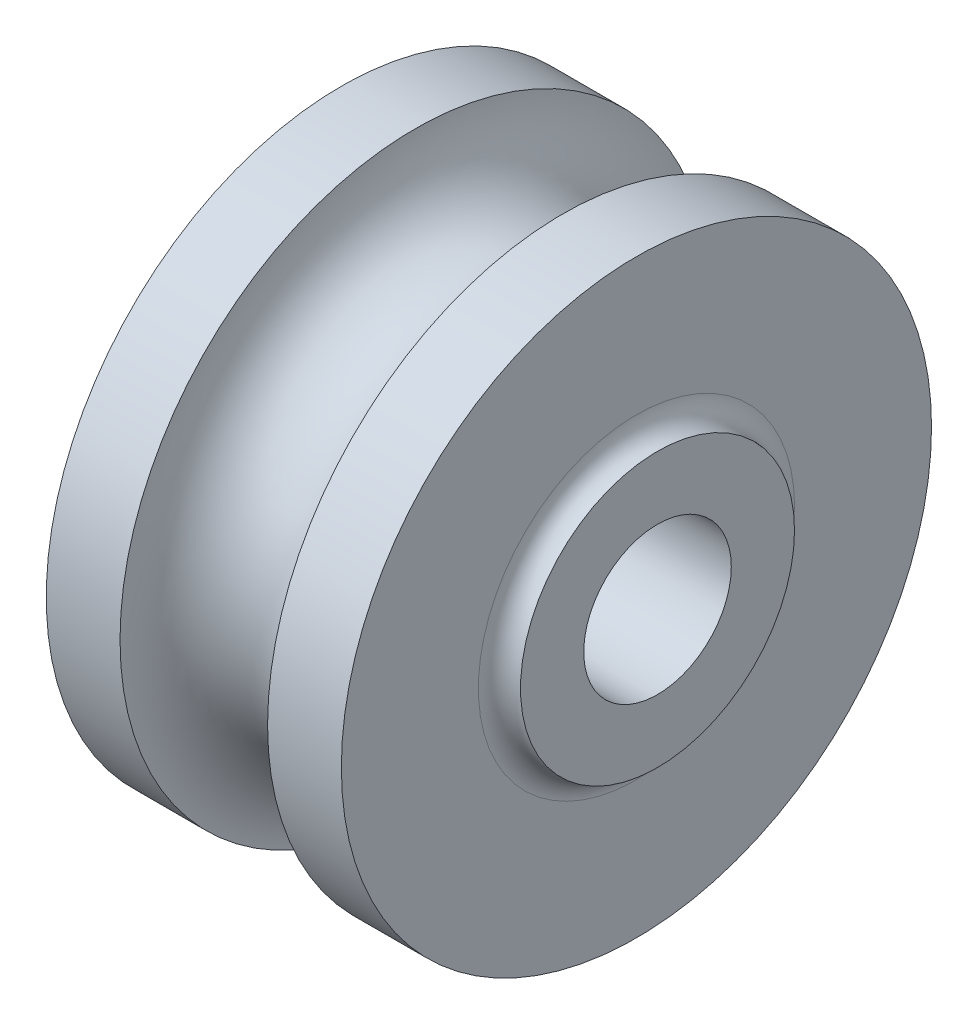
ISO-10303-21;
HEADER;
FILE_DESCRIPTION(('STEP AP214'),'2;1');
FILE_NAME('part.step','',(''),(''),'','','');
FILE_SCHEMA(('AUTOMOTIVE_DESIGN { 1 0 10303 214 1 1 1 1 }'));
ENDSEC;
DATA;
#1=APPLICATION_CONTEXT('core data for automotive mechanical design processes');
#2=APPLICATION_PROTOCOL_DEFINITION('international standard','automotive_design',2000,#1);
#3=PRODUCT_CONTEXT('',#1,'mechanical');
#4=PRODUCT('Part','Part','',(#3));
#5=PRODUCT_RELATED_PRODUCT_CATEGORY('part','',(#4));
#6=PRODUCT_DEFINITION_FORMATION('','',#4);
#7=PRODUCT_DEFINITION_CONTEXT('part definition',#1,'design');
#8=PRODUCT_DEFINITION('design','',#6,#7);
#9=PRODUCT_DEFINITION_SHAPE('','',#8);
#10=(LENGTH_UNIT() NAMED_UNIT(*) SI_UNIT(.MILLI.,.METRE.));
#11=(NAMED_UNIT(*) PLANE_ANGLE_UNIT() SI_UNIT($,.RADIAN.));
#12=(NAMED_UNIT(*) SI_UNIT($,.STERADIAN.) SOLID_ANGLE_UNIT());
#13=UNCERTAINTY_MEASURE_WITH_UNIT(LENGTH_MEASURE(1.E-05),#10,'distance_accuracy_value','');
#14=(GEOMETRIC_REPRESENTATION_CONTEXT(3) GLOBAL_UNCERTAINTY_ASSIGNED_CONTEXT((#13)) GLOBAL_UNIT_ASSIGNED_CONTEXT((#10,
#11,#12)) REPRESENTATION_CONTEXT('',''));
#15=CARTESIAN_POINT('',(0.,0.,0.));
#16=DIRECTION('',(0.,0.,1.));
#17=DIRECTION('',(1.,0.,0.));
#18=AXIS2_PLACEMENT_3D('',#15,#16,#17);
#19=CARTESIAN_POINT('',(14.,0.,0.));
#20=DIRECTION('',(-1.,0.,0.));
#21=DIRECTION('',(0.,0.,1.));
#22=AXIS2_PLACEMENT_3D('',#19,#20,#21);
#23=CYLINDRICAL_SURFACE('',#22,28.);
#24=CARTESIAN_POINT('',(-14.,0.,0.));
#25=DIRECTION('',(1.,0.,0.));
#26=DIRECTION('',(0.,0.,-1.));
#27=AXIS2_PLACEMENT_3D('',#24,#25,#26);
#28=CIRCLE('',#27,28.);
#29=CARTESIAN_POINT('',(-14.,0.,-28.));
#30=VERTEX_POINT('',#29);
#31=EDGE_CURVE('E78',#30,#30,#28,.T.);
#32=ORIENTED_EDGE('',*,*,#31,.T.);
#33=EDGE_LOOP('',(#32));
#34=FACE_BOUND('',#33,.T.);
#35=CARTESIAN_POINT('',(-7.,0.,0.));
#36=DIRECTION('',(1.,0.,0.));
#37=DIRECTION('',(0.,0.,-1.));
#38=AXIS2_PLACEMENT_3D('',#35,#36,#37);
#39=CIRCLE('',#38,28.);
#40=CARTESIAN_POINT('',(-7.,0.,-28.));
#41=VERTEX_POINT('',#40);
#42=EDGE_CURVE('E43',#41,#41,#39,.T.);
#43=ORIENTED_EDGE('',*,*,#42,.F.);
#44=EDGE_LOOP('',(#43));
#45=FACE_BOUND('',#44,.T.);
#46=ADVANCED_FACE('F39',(#34,#45),#23,.T.);
#47=CARTESIAN_POINT('',(14.,0.,0.));
#48=DIRECTION('',(1.,0.,0.));
#49=DIRECTION('',(0.,0.,-1.));
#50=AXIS2_PLACEMENT_3D('',#47,#48,#49);
#51=CIRCLE('',#50,28.);
#52=CARTESIAN_POINT('',(14.,0.,-28.));
#53=VERTEX_POINT('',#52);
#54=EDGE_CURVE('E55',#53,#53,#51,.T.);
#55=ORIENTED_EDGE('',*,*,#54,.F.);
#56=EDGE_LOOP('',(#55));
#57=FACE_BOUND('',#56,.T.);
#58=CARTESIAN_POINT('',(7.,0.,0.));
#59=DIRECTION('',(-1.,0.,0.));
#60=DIRECTION('',(0.,0.,1.));
#61=AXIS2_PLACEMENT_3D('',#58,#59,#60);
#62=CIRCLE('',#61,28.);
#63=CARTESIAN_POINT('',(7.,0.,28.));
#64=VERTEX_POINT('',#63);
#65=EDGE_CURVE('E54',#64,#64,#62,.T.);
#66=ORIENTED_EDGE('',*,*,#65,.F.);
#67=EDGE_LOOP('',(#66));
#68=FACE_BOUND('',#67,.T.);
#69=ADVANCED_FACE('F102',(#57,#68),#23,.T.);
#70=CARTESIAN_POINT('',(14.,0.,0.));
#71=DIRECTION('',(1.,0.,0.));
#72=DIRECTION('',(0.,0.,-1.));
#73=AXIS2_PLACEMENT_3D('',#70,#71,#72);
#74=PLANE('',#73);
#75=CARTESIAN_POINT('',(14.,0.,0.));
#76=DIRECTION('',(1.,0.,0.));
#77=DIRECTION('',(0.,0.,-1.));
#78=AXIS2_PLACEMENT_3D('',#75,#76,#77);
#79=CIRCLE('',#78,15.);
#80=CARTESIAN_POINT('',(14.,0.,-15.));
#81=VERTEX_POINT('',#80);
#82=EDGE_CURVE('E50',#81,#81,#79,.F.);
#83=ORIENTED_EDGE('',*,*,#82,.T.);
#84=EDGE_LOOP('',(#83));
#85=FACE_BOUND('',#84,.T.);
#86=ORIENTED_EDGE('',*,*,#54,.T.);
#87=EDGE_LOOP('',(#86));
#88=FACE_BOUND('',#87,.T.);
#89=ADVANCED_FACE('F109',(#85,#88),#74,.T.);
#90=CARTESIAN_POINT('',(-14.,0.,0.));
#91=DIRECTION('',(1.,0.,0.));
#92=DIRECTION('',(0.,0.,-1.));
#93=AXIS2_PLACEMENT_3D('',#90,#91,#92);
#94=PLANE('',#93);
#95=CARTESIAN_POINT('',(-14.,0.,0.));
#96=DIRECTION('',(1.,0.,0.));
#97=DIRECTION('',(0.,0.,-1.));
#98=AXIS2_PLACEMENT_3D('',#95,#96,#97);
#99=CIRCLE('',#98,15.);
#100=CARTESIAN_POINT('',(-14.,0.,-15.));
#101=VERTEX_POINT('',#100);
#102=EDGE_CURVE('E10',#101,#101,#99,.T.);
#103=ORIENTED_EDGE('',*,*,#102,.T.);
#104=EDGE_LOOP('',(#103));
#105=FACE_BOUND('',#104,.T.);
#106=ORIENTED_EDGE('',*,*,#31,.F.);
#107=EDGE_LOOP('',(#106));
#108=FACE_BOUND('',#107,.T.);
#109=ADVANCED_FACE('F111',(#105,#108),#94,.F.);
#110=CARTESIAN_POINT('',(-16.,0.,0.));
#111=DIRECTION('',(1.,0.,0.));
#112=DIRECTION('',(0.,0.,-1.));
#113=AXIS2_PLACEMENT_3D('',#110,#111,#112);
#114=PLANE('',#113);
#115=CARTESIAN_POINT('',(-16.,0.,0.));
#116=DIRECTION('',(1.,0.,0.));
#117=DIRECTION('',(0.,0.,-1.));
#118=AXIS2_PLACEMENT_3D('',#115,#116,#117);
#119=CIRCLE('',#118,7.);
#120=CARTESIAN_POINT('',(-16.,0.,-7.));
#121=VERTEX_POINT('',#120);
#122=EDGE_CURVE('E58',#121,#121,#119,.T.);
#123=ORIENTED_EDGE('',*,*,#122,.T.);
#124=EDGE_LOOP('',(#123));
#125=FACE_BOUND('',#124,.T.);
#126=CARTESIAN_POINT('',(-16.,0.,0.));
#127=DIRECTION('',(1.,0.,0.));
#128=DIRECTION('',(0.,0.,-1.));
#129=AXIS2_PLACEMENT_3D('',#126,#127,#128);
#130=CIRCLE('',#129,13.);
#131=CARTESIAN_POINT('',(-16.,0.,-13.));
#132=VERTEX_POINT('',#131);
#133=EDGE_CURVE('E64',#132,#132,#130,.T.);
#134=ORIENTED_EDGE('',*,*,#133,.F.);
#135=EDGE_LOOP('',(#134));
#136=FACE_BOUND('',#135,.T.);
#137=ADVANCED_FACE('F98',(#125,#136),#114,.F.);
#138=CARTESIAN_POINT('',(14.,0.,0.));
#139=DIRECTION('',(-1.,0.,0.));
#140=DIRECTION('',(0.,0.,1.));
#141=AXIS2_PLACEMENT_3D('',#138,#139,#140);
#142=CYLINDRICAL_SURFACE('',#141,7.);
#143=ORIENTED_EDGE('',*,*,#122,.F.);
#144=EDGE_LOOP('',(#143));
#145=FACE_BOUND('',#144,.T.);
#146=CARTESIAN_POINT('',(16.,0.,0.));
#147=DIRECTION('',(1.,0.,0.));
#148=DIRECTION('',(0.,0.,-1.));
#149=AXIS2_PLACEMENT_3D('',#146,#147,#148);
#150=CIRCLE('',#149,7.);
#151=CARTESIAN_POINT('',(16.,0.,-7.));
#152=VERTEX_POINT('',#151);
#153=EDGE_CURVE('E70',#152,#152,#150,.T.);
#154=ORIENTED_EDGE('',*,*,#153,.T.);
#155=EDGE_LOOP('',(#154));
#156=FACE_BOUND('',#155,.T.);
#157=ADVANCED_FACE('F88',(#145,#156),#142,.F.);
#158=CARTESIAN_POINT('',(16.,0.,0.));
#159=DIRECTION('',(1.,0.,0.));
#160=DIRECTION('',(0.,0.,-1.));
#161=AXIS2_PLACEMENT_3D('',#158,#159,#160);
#162=PLANE('',#161);
#163=ORIENTED_EDGE('',*,*,#153,.F.);
#164=EDGE_LOOP('',(#163));
#165=FACE_BOUND('',#164,.T.);
#166=CARTESIAN_POINT('',(16.,0.,0.));
#167=DIRECTION('',(1.,0.,0.));
#168=DIRECTION('',(0.,0.,-1.));
#169=AXIS2_PLACEMENT_3D('',#166,#167,#168);
#170=CIRCLE('',#169,13.);
#171=CARTESIAN_POINT('',(16.,0.,-13.));
#172=VERTEX_POINT('',#171);
#173=EDGE_CURVE('E75',#172,#172,#170,.T.);
#174=ORIENTED_EDGE('',*,*,#173,.T.);
#175=EDGE_LOOP('',(#174));
#176=FACE_BOUND('',#175,.T.);
#177=ADVANCED_FACE('F86',(#165,#176),#162,.T.);
#178=CARTESIAN_POINT('',(16.,0.,0.));
#179=DIRECTION('',(1.,0.,0.));
#180=DIRECTION('',(0.,0.,-1.));
#181=AXIS2_PLACEMENT_3D('',#178,#179,#180);
#182=TOROIDAL_SURFACE('',#181,15.,2.);
#183=ORIENTED_EDGE('',*,*,#173,.F.);
#184=EDGE_LOOP('',(#183));
#185=FACE_BOUND('',#184,.T.);
#186=ORIENTED_EDGE('',*,*,#82,.F.);
#187=EDGE_LOOP('',(#186));
#188=FACE_BOUND('',#187,.T.);
#189=ADVANCED_FACE('F89',(#185,#188),#182,.F.);
#190=CARTESIAN_POINT('',(-16.,0.,0.));
#191=DIRECTION('',(1.,0.,0.));
#192=DIRECTION('',(0.,0.,-1.));
#193=AXIS2_PLACEMENT_3D('',#190,#191,#192);
#194=TOROIDAL_SURFACE('',#193,15.,2.);
#195=ORIENTED_EDGE('',*,*,#102,.F.);
#196=EDGE_LOOP('',(#195));
#197=FACE_BOUND('',#196,.T.);
#198=ORIENTED_EDGE('',*,*,#133,.T.);
#199=EDGE_LOOP('',(#198));
#200=FACE_BOUND('',#199,.T.);
#201=ADVANCED_FACE('F41',(#197,#200),#194,.F.);
#202=CARTESIAN_POINT('',(0.,0.,0.));
#203=DIRECTION('',(-1.,0.,0.));
#204=DIRECTION('',(0.,0.,1.));
#205=AXIS2_PLACEMENT_3D('',#202,#203,#204);
#206=TOROIDAL_SURFACE('',#205,28.,7.);
#207=ORIENTED_EDGE('',*,*,#65,.T.);
#208=EDGE_LOOP('',(#207));
#209=FACE_BOUND('',#208,.T.);
#210=ORIENTED_EDGE('',*,*,#42,.T.);
#211=EDGE_LOOP('',(#210));
#212=FACE_BOUND('',#211,.T.);
#213=ADVANCED_FACE('F125',(#209,#212),#206,.F.);
#214=CLOSED_SHELL('',(#46,#69,#89,#109,#137,#157,#177,#189,#201,#213));
#215=MANIFOLD_SOLID_BREP('B2',#214);
#216=ADVANCED_BREP_SHAPE_REPRESENTATION('',(#18,#215),#14);
#217=SHAPE_DEFINITION_REPRESENTATION(#9,#216);
ENDSEC;
END-ISO-10303-21;
